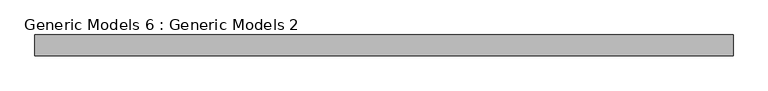
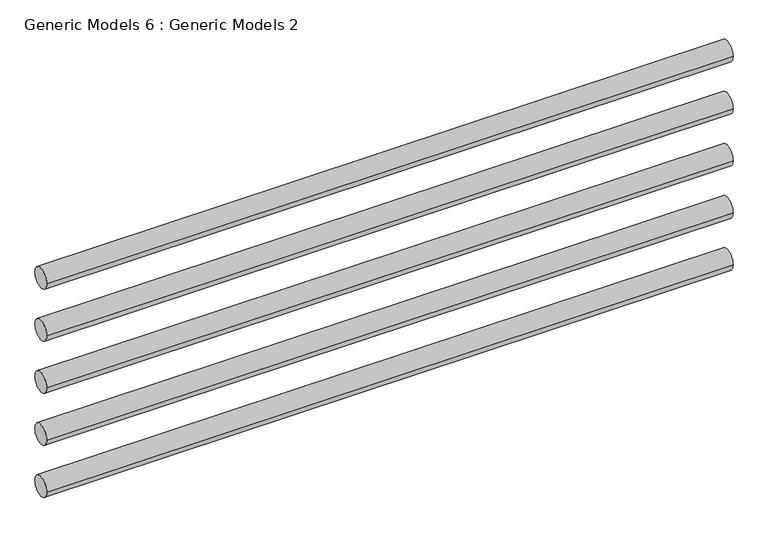
"""IFC4 building model written with IfcOpenShell, lengths in millimetres: proxy geometry, Generic Models 6 : Generic Models 2."""

from ifc_helpers import new_model, si_unit, point, frame, frame_2d, origin, place, context, project, spatial, circle_curve, trimmed, segment, composite_curve, outline, extrude, source, transform, mapped, element, save


def generic_models_6_generic_models_2_9af304e7(model_context):
    return source(origin(), model_context, "Body", "SweptSolid", [
        extrude(outline(composite_curve([segment(trimmed(circle_curve(frame_2d((-4479.5968048, 7808.1544804)), 38.1), [point((-4517.6968048, 7808.1544804))], [point((-4441.4968048, 7808.1544804))], False, "CARTESIAN"), True, "CONTINUOUS"), segment(trimmed(circle_curve(frame_2d((-4479.5968048, 7808.1544804)), 38.1), [point((-4441.4968048, 7808.1544804))], [point((-4517.6968048, 7808.1544804))], False, "CARTESIAN"), True, "CONTINUOUS")], self_intersect=False)), frame((-14722.761259, 0.0, 0.0), z_axis=(1.0, 0.0, 0.0), x_axis=(0.0, 1.0, 0.0)), (0.0, 0.0, 1.0), 2531.6821699),
        extrude(outline(composite_curve([segment(trimmed(circle_curve(frame_2d((-4479.5968048, 7604.9544804)), 38.1), [point((-4517.6968048, 7604.9544804))], [point((-4441.4968048, 7604.9544804))], False, "CARTESIAN"), True, "CONTINUOUS"), segment(trimmed(circle_curve(frame_2d((-4479.5968048, 7604.9544804)), 38.1), [point((-4441.4968048, 7604.9544804))], [point((-4517.6968048, 7604.9544804))], False, "CARTESIAN"), True, "CONTINUOUS")], self_intersect=False)), frame((-14722.761259, 0.0, 0.0), z_axis=(1.0, 0.0, 0.0), x_axis=(0.0, 1.0, 0.0)), (0.0, 0.0, 1.0), 2531.6821699),
        extrude(outline(composite_curve([segment(trimmed(circle_curve(frame_2d((-4479.5968048, 7401.7544804)), 38.1), [point((-4517.6968048, 7401.7544804))], [point((-4441.4968048, 7401.7544804))], False, "CARTESIAN"), True, "CONTINUOUS"), segment(trimmed(circle_curve(frame_2d((-4479.5968048, 7401.7544804)), 38.1), [point((-4441.4968048, 7401.7544804))], [point((-4517.6968048, 7401.7544804))], False, "CARTESIAN"), True, "CONTINUOUS")], self_intersect=False)), frame((-14722.761259, 0.0, 0.0), z_axis=(1.0, 0.0, 0.0), x_axis=(0.0, 1.0, 0.0)), (0.0, 0.0, 1.0), 2531.6821699),
        extrude(outline(composite_curve([segment(trimmed(circle_curve(frame_2d((-4479.5968048, 7198.5544804)), 38.1), [point((-4517.6968048, 7198.5544804))], [point((-4441.4968048, 7198.5544804))], False, "CARTESIAN"), True, "CONTINUOUS"), segment(trimmed(circle_curve(frame_2d((-4479.5968048, 7198.5544804)), 38.1), [point((-4441.4968048, 7198.5544804))], [point((-4517.6968048, 7198.5544804))], False, "CARTESIAN"), True, "CONTINUOUS")], self_intersect=False)), frame((-14722.761259, 0.0, 0.0), z_axis=(1.0, 0.0, 0.0), x_axis=(0.0, 1.0, 0.0)), (0.0, 0.0, 1.0), 2531.6821699),
        extrude(outline(composite_curve([segment(trimmed(circle_curve(frame_2d((-4479.5968048, 6995.3544804)), 38.1), [point((-4517.6968048, 6995.3544804))], [point((-4441.4968048, 6995.3544804))], False, "CARTESIAN"), True, "CONTINUOUS"), segment(trimmed(circle_curve(frame_2d((-4479.5968048, 6995.3544804)), 38.1), [point((-4441.4968048, 6995.3544804))], [point((-4517.6968048, 6995.3544804))], False, "CARTESIAN"), True, "CONTINUOUS")], self_intersect=False)), frame((-14722.761259, 0.0, 0.0), z_axis=(1.0, 0.0, 0.0), x_axis=(0.0, 1.0, 0.0)), (0.0, 0.0, 1.0), 2531.6821699),
    ])


if __name__ == "__main__":
    model = new_model("IFC4")
    model_context = context("Model", 3, world=origin())
    ifc_project = project(units=[si_unit("LENGTHUNIT", "METRE", prefix="MILLI")], contexts=[model_context])
    site = spatial("IfcSite", under=ifc_project)
    building = spatial("IfcBuilding", under=site)
    placement = place(None, origin())
    generic_models_6_generic_models_2_shape = generic_models_6_generic_models_2_9af304e7(model_context)
    element("IfcBuildingElementProxy", 1, Name="Generic Models 6 : Generic Models 2", ObjectType="Generic Models 6 : Generic Models 2", at=placement, inside=building, context=model_context, shape_type="MappedRepresentation", body=[
        mapped(generic_models_6_generic_models_2_shape, transform((0.0, 0.0, 0.0), x_axis=(1.0, 0.0, 0.0), y_axis=(0.0, 1.0, 0.0), z_axis=(0.0, 0.0, 1.0))),
    ])
    save(model, "model.ifc")
